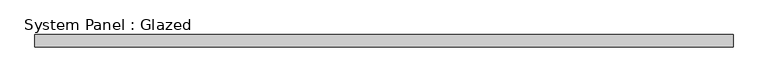
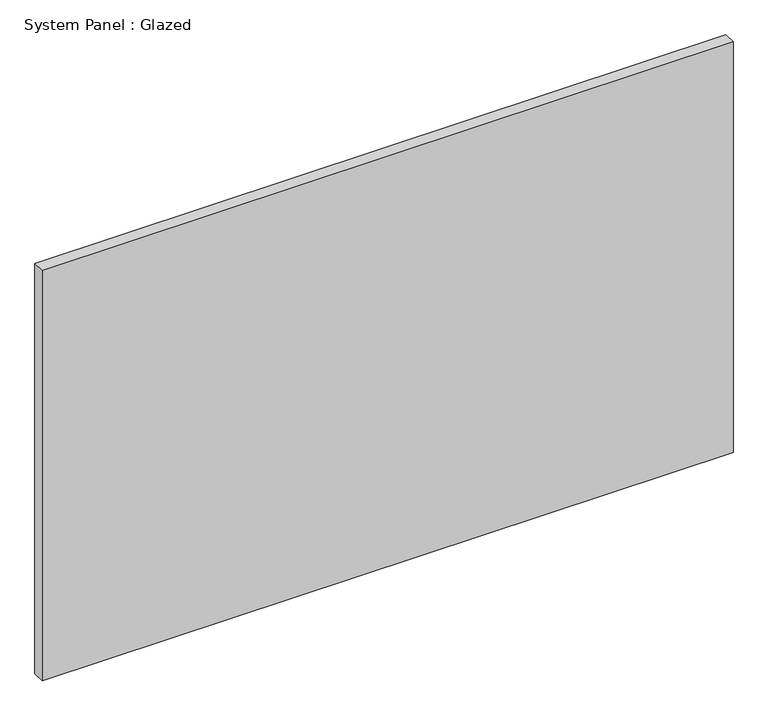
"""IFC4 building model written with IfcOpenShell, lengths in millimetres: plate geometry, System Panel : Glazed."""

from ifc_helpers import new_model, si_unit, origin, origin_with_axes, place, context, project, spatial, polyline, outline, extrude, source, transform, mapped, element, save


def system_panel_glazed_7b3c61a9(model_context):
    return source(origin(), model_context, "Body", "SweptSolid", [
        extrude(outline(polyline([(714.375, 19.05), (-714.375, 19.05), (-714.375, 44.45), (714.375, 44.45), (714.375, 19.05)])), origin_with_axes(), (0.0, 0.0, 1.0), 897.5064813),
    ])


if __name__ == "__main__":
    model = new_model("IFC4")
    model_context = context("Model", 3, world=origin())
    ifc_project = project(units=[si_unit("LENGTHUNIT", "METRE", prefix="MILLI")], contexts=[model_context])
    site = spatial("IfcSite", under=ifc_project)
    building = spatial("IfcBuilding", under=site)
    placement = place(None, origin())
    system_panel_glazed_shape = system_panel_glazed_7b3c61a9(model_context)
    element("IfcPlate", 1, ObjectType="System Panel : Glazed", at=placement, inside=building, context=model_context, shape_type="MappedRepresentation", body=[
        mapped(system_panel_glazed_shape, transform((0.0, 0.0, 0.0), x_axis=(1.0, 0.0, 0.0), y_axis=(0.0, 1.0, 0.0), z_axis=(0.0, 0.0, 1.0))),
    ])
    save(model, "model.ifc")

# Revit data of these elements
# Type "System Panel : Glazed"
#   Construction Type Id = "GSP4R"
#   Analytic Construction = "1/8 in Pilkington single glazing"
#   Visual Light Transmittance = 0.9
#   Solar Heat Gain Coefficient = 0.86
#   Heat Transfer Coefficient (U) = 1.18115 BTU/(h·ft²·°F)
#   Define Thermal Properties by = 1
# Element 1 (IfcPlate, "System Panel : Glazed")
#   Materials on its faces: "Glass"
# Materials
#   "Glass": class "Glass", colour RGB 0 128 192, transparency 0.75, Description = "Soda Lime Glass", Cost = 0
